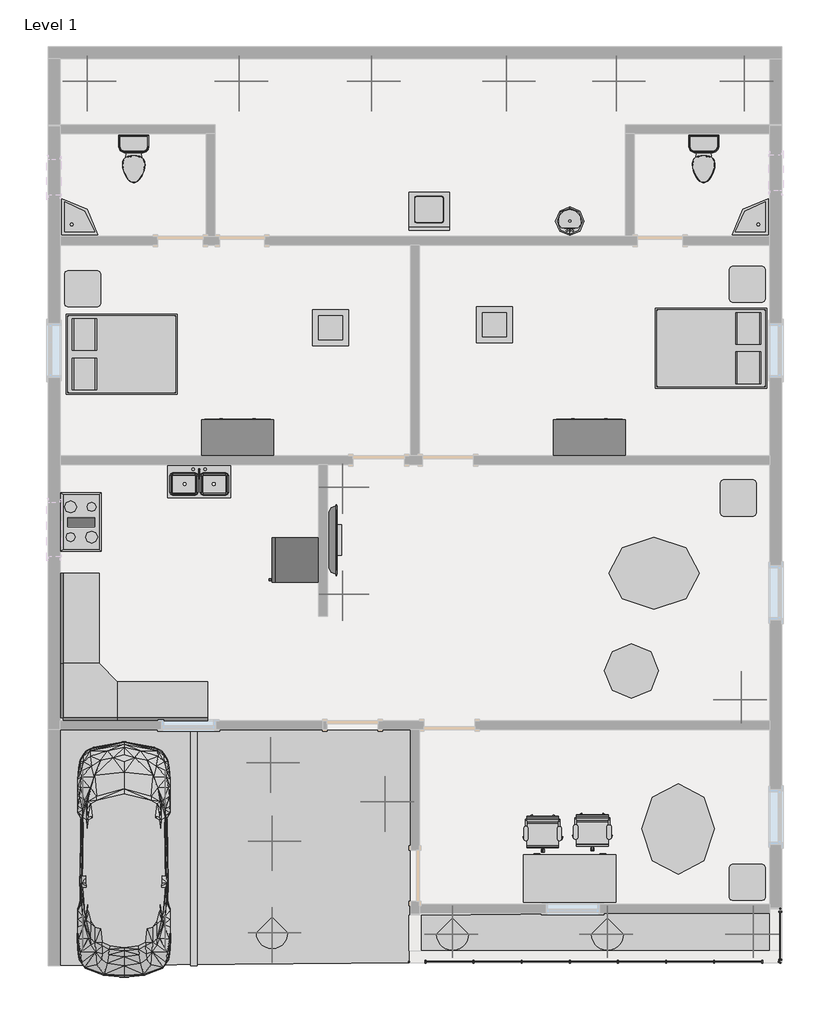
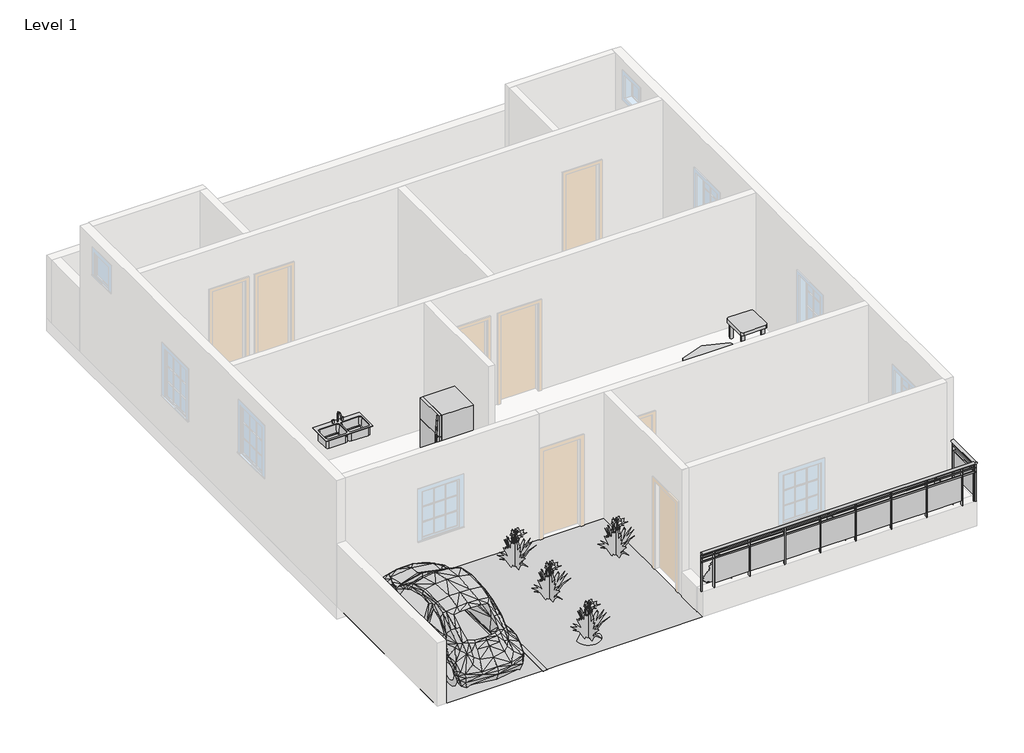
# One storey, part 2 of 2: 18 furniture elements, 16 geographic elements, 9 flow terminals, 7 proxies, 2 railings.
"""IFC4 building model written with IfcOpenShell, lengths in millimetres."""

from ifc_helpers import new_model, si_unit, point, frame, origin, place, context, project, spatial, polyline, ellipse_curve, trimmed, outline, extrude, triangles, transform, mapped, element, save
from ifc_brep_helpers import plane_surface, extruded_surface, advanced_brep
from components import proxy_bb1e6e30, m_rpc_beetle_m_rpc_beetle_b6d71803, parking_space_9_x_18_90_deg_c935943f, proxy_a13a33b2, proxy_718fa39f, flow_terminal_2b63360b, flow_terminal_accce45a, flow_terminal_bd5cdcf8, flow_terminal_a53be723, flow_terminal_d49f872f, toilet_domestic_3d_toilet_domestic_3d_f7549cf7, toilet_domestic_3d_toilet_domestic_3d_183bbd19, furniture_c8abb964, chair_task_arms_chair_task_arms_fa5a08ef, furniture_072f6425, furniture_9fa109b2, furniture_d9bcc661, furniture_b5c51a22, furniture_905aceb5, furniture_743965d2, furniture_5d68651d, furniture_45e3acac, rpc_plant_tropical_55f6ff97, rpc_plant_tropical_dagger_2_80c14bd7, rpc_plant_tropical_jungle_flame_3_9c4808c2

model = new_model("IFC4")

# Units and contexts
model_context = context("Model", 3, world=origin())
ifc_project = project(units=[si_unit("LENGTHUNIT", "METRE", prefix="MILLI")], contexts=[model_context])

# Site, building, storey
site = spatial("IfcSite", under=ifc_project)
building = spatial("IfcBuilding", under=site)
storey = spatial("IfcBuildingStorey", under=building, Name="Level 1", Elevation=0.0)

# Proxies
placement = place(None, origin())
element("IfcBuildingElementProxy", 1, Name="Building Element Proxy", at=placement, inside=storey, context=model_context, shape_type="Tessellation", body=[
    triangles([(-12787.9240906, 4557.2232857, 0.0), (-6666.5238968, 4557.2232857, 0.0), (-6679.223703, 620.2234068, 0.0), (-12787.9961792, 723.5583784, 0.0), (-7358.6740906, 4658.8234795, 0.0), (-6926.873703, 4658.8234795, 0.0), (-12584.723703, 569.4234189, 0.0)], [[4, 7, 1], [1, 7, 5], [3, 2, 5], [6, 5, 2], [3, 5, 7]], closed=False),
])
element("IfcBuildingElementProxy", 2, Name="Building Element Proxy", at=placement, inside=storey, context=model_context, shape_type="Tessellation", body=[
    triangles([(-6488.723703, 1420.3234795, 0.0), (-6488.723703, 823.423431, 0.0), (-595.9238726, 1458.4234795, 0.0), (-595.9238726, 823.423431, 0.0), (-3122.7224739, 1458.4234795, 0.0)], [[1, 2, 5], [5, 4, 3], [4, 5, 2]], closed=False),
])
proxy_shape = proxy_bb1e6e30(model_context)
element("IfcBuildingElementProxy", 3, Name="Cook Top-4 Unit : 36\" x 20\"", ObjectType="Cook Top-4 Unit : 36\" x 20\"", at=placement, inside=storey, context=model_context, shape_type="MappedRepresentation", body=[
    mapped(proxy_shape, transform((-12229.1238552, 8062.4234128, 0.0), x_axis=(0.0, 1.0000000000000002, 0.0), y_axis=(-1.0000000000000002, 0.0, 0.0), z_axis=(0.0, 0.0, 1.0))),
])
m_rpc_beetle_m_rpc_beetle_shape = m_rpc_beetle_m_rpc_beetle_b6d71803(model_context)
element("IfcBuildingElementProxy", 4, Name="M_RPC Beetle : M_RPC Beetle", ObjectType="M_RPC Beetle : M_RPC Beetle", at=placement, inside=storey, context=model_context, shape_type="MappedRepresentation", body=[
    mapped(m_rpc_beetle_m_rpc_beetle_shape, transform((-11505.2238552, 1128.2234128, 0.0), x_axis=(1.0, 0.0, 0.0), y_axis=(0.0, 1.0, 0.0), z_axis=(0.0, 0.0, 1.0))),
])
parking_space_9_x_18_90_deg_shape = parking_space_9_x_18_90_deg_c935943f(model_context)
element("IfcBuildingElementProxy", 5, Name="Parking Space : 9' x 18' - 90 deg", ObjectType="Parking Space : 9' x 18' - 90 deg", at=placement, inside=storey, context=model_context, shape_type="MappedRepresentation", body=[
    mapped(parking_space_9_x_18_90_deg_shape, transform((-10324.1238552, 569.4234128, 0.0), x_axis=(-1.0000000000000004, 0.0, 0.0), y_axis=(0.0, -1.0000000000000004, 0.0), z_axis=(0.0, 0.0, 1.0))),
])
proxy_2_shape = proxy_a13a33b2(model_context)
element("IfcBuildingElementProxy", 6, Name="Refrigerator : 30\" x 32\" RH", ObjectType="Refrigerator : 30\" x 32\" RH", at=placement, inside=storey, context=model_context, shape_type="MappedRepresentation", body=[
    mapped(proxy_2_shape, transform((-8588.9863552, 7419.8744413, 0.0), x_axis=(0.0, -1.0000000000000007, 0.0), y_axis=(1.0000000000000007, 0.0, 0.0), z_axis=(0.0, 0.0, 1.0))),
])
proxy_3_shape = proxy_718fa39f(model_context)
element("IfcBuildingElementProxy", 7, Name="Washer : 27\" x 25\" x 35\"", ObjectType="Washer : 27\" x 25\" x 35\"", at=placement, inside=storey, context=model_context, shape_type="MappedRepresentation", body=[
    mapped(proxy_3_shape, transform((-5931.2413237, 13587.173848, 0.0), x_axis=(-1.0000000000000004, 0.0, 0.0), y_axis=(0.0, -1.0000000000000004, 0.0), z_axis=(0.0, 0.0, 1.0))),
])

# Flow terminals
flow_terminal_shape = flow_terminal_2b63360b(model_context)
element("IfcFlowTerminal", 8, ObjectType="Floor Drain - Rectangular : 5\"x5\" Strainer - 2\" Drain", at=placement, inside=storey, context=model_context, shape_type="MappedRepresentation", body=[
    mapped(flow_terminal_shape, transform((-4710.7238552, 13066.2234128, 0.0), x_axis=(1.0, 0.0, 0.0), y_axis=(0.0, 1.0, 0.0), z_axis=(0.0, 0.0, 1.0))),
])
flow_terminal_2_shape = flow_terminal_accce45a(model_context)
element("IfcFlowTerminal", 9, ObjectType="Floor Drain - Round : 5\" Strainer - 2\" Drain", at=placement, inside=storey, context=model_context, shape_type="MappedRepresentation", body=[
    mapped(flow_terminal_2_shape, transform((-10425.7238552, 14361.6234128, 0.0), x_axis=(1.0, 0.0, 0.0), y_axis=(0.0, 1.0, 0.0), z_axis=(0.0, 0.0, 1.0))),
])
element("IfcFlowTerminal", 10, ObjectType="Floor Drain - Round : 5\" Strainer - 2\" Drain", at=placement, inside=storey, context=model_context, shape_type="MappedRepresentation", body=[
    mapped(flow_terminal_2_shape, transform((-2627.9238552, 14412.4234128, 0.0), x_axis=(1.0, 0.0, 0.0), y_axis=(0.0, 1.0, 0.0), z_axis=(0.0, 0.0, 1.0))),
])
flow_terminal_3_shape = flow_terminal_bd5cdcf8(model_context)
element("IfcFlowTerminal", 11, ObjectType="Sink - Corner Floor : 24\"", at=placement, inside=storey, context=model_context, shape_type="MappedRepresentation", body=[
    mapped(flow_terminal_3_shape, transform((-12559.3238552, 12913.8234128, 609.6), x_axis=(1.0, 0.0, 0.0), y_axis=(0.0, 1.0, 0.0), z_axis=(0.0, 0.0, 1.0))),
])
element("IfcFlowTerminal", 12, ObjectType="Sink - Corner Floor : 24\"", at=placement, inside=storey, context=model_context, shape_type="MappedRepresentation", body=[
    mapped(flow_terminal_3_shape, transform((-621.3238552, 12913.8234128, 609.6), x_axis=(0.0, 1.0, 0.0), y_axis=(-1.0, 0.0, 0.0), z_axis=(0.0, 0.0, 1.0))),
])
flow_terminal_4_shape = flow_terminal_a53be723(model_context)
element("IfcFlowTerminal", 13, ObjectType="Sink Kitchen-Double : 42\" x 21\"", at=placement, inside=storey, context=model_context, shape_type="MappedRepresentation", body=[
    mapped(flow_terminal_4_shape, transform((-10250.9130958, 8739.5280117, 0.0), x_axis=(1.0, 0.0, 0.0), y_axis=(0.0, 1.0, 0.0), z_axis=(0.0, 0.0, 1.0))),
])
flow_terminal_5_shape = flow_terminal_d49f872f(model_context)
element("IfcFlowTerminal", 14, ObjectType="Sink Vanity-Round : 19\" x 19\"", at=placement, inside=storey, context=model_context, shape_type="MappedRepresentation", body=[
    mapped(flow_terminal_5_shape, transform((-3877.4721147, 13227.1912438, 304.8), x_axis=(-1.0000000000000004, 0.0, 0.0), y_axis=(0.0, -1.0000000000000004, 0.0), z_axis=(0.0, 0.0, 1.0))),
])
toilet_domestic_3d_toilet_domestic_3d_shape = toilet_domestic_3d_toilet_domestic_3d_f7549cf7(model_context)
toilet_domestic_3d_toilet_domestic_3d_2_shape = toilet_domestic_3d_toilet_domestic_3d_183bbd19(model_context)
element("IfcFlowTerminal", 15, ObjectType="Toilet-Domestic-3D : Toilet-Domestic-3D", at=placement, inside=storey, context=model_context, shape_type="MappedRepresentation", body=[
    mapped(toilet_domestic_3d_toilet_domestic_3d_shape, transform((-11340.1238552, 14095.5273855, 0.0), x_axis=(1.0, 0.0, 0.0), y_axis=(0.0, 1.0, 0.0), z_axis=(0.0, 0.0, 1.0))),
    mapped(toilet_domestic_3d_toilet_domestic_3d_2_shape, transform((-11340.1238552, 14095.5273855, 0.0), x_axis=(1.0, 0.0, 0.0), y_axis=(0.0, 1.0, 0.0), z_axis=(0.0, 0.0, 1.0))),
])
element("IfcFlowTerminal", 16, ObjectType="Toilet-Domestic-3D : Toilet-Domestic-3D", at=placement, inside=storey, context=model_context, shape_type="MappedRepresentation", body=[
    mapped(toilet_domestic_3d_toilet_domestic_3d_shape, transform((-1713.5238552, 14095.5273855, 0.0), x_axis=(1.0, 0.0, 0.0), y_axis=(0.0, 1.0, 0.0), z_axis=(0.0, 0.0, 1.0))),
    mapped(toilet_domestic_3d_toilet_domestic_3d_2_shape, transform((-1713.5238552, 14095.5273855, 0.0), x_axis=(1.0, 0.0, 0.0), y_axis=(0.0, 1.0, 0.0), z_axis=(0.0, 0.0, 1.0))),
])

# Furniture
furniture_shape = furniture_c8abb964(model_context)
element("IfcFurniture", 17, ObjectType="Bed-Box : Double 53\" x 74\"", at=placement, inside=storey, context=model_context, shape_type="MappedRepresentation", body=[
    mapped(furniture_shape, transform((-11777.7533634, 10555.3709538, 0.0), x_axis=(0.0, 1.0, 0.0), y_axis=(-1.0, 0.0, 0.0), z_axis=(0.0, 0.0, 1.0))),
])
element("IfcFurniture", 18, ObjectType="Bed-Box : Double 53\" x 74\"", at=placement, inside=storey, context=model_context, shape_type="MappedRepresentation", body=[
    mapped(furniture_shape, transform((-1352.094347, 11335.2758718, 0.0), x_axis=(0.0, -1.0, 0.0), y_axis=(1.0, 0.0, 0.0), z_axis=(0.0, 0.0, 1.0))),
])
chair_task_arms_chair_task_arms_shape = chair_task_arms_chair_task_arms_fa5a08ef(model_context)
element("IfcFurniture", 19, ObjectType="Chair-Task Arms : Chair-Task Arms", at=placement, inside=storey, context=model_context, shape_type="MappedRepresentation", body=[
    mapped(chair_task_arms_chair_task_arms_shape, transform((-4290.3330355, 2848.9693144, 0.0), x_axis=(-1.000000000000001, 0.0, 0.0), y_axis=(0.0, -1.000000000000001, 0.0), z_axis=(0.0, 0.0, 1.0))),
])
element("IfcFurniture", 20, ObjectType="Chair-Task Arms : Chair-Task Arms", at=placement, inside=storey, context=model_context, shape_type="MappedRepresentation", body=[
    mapped(chair_task_arms_chair_task_arms_shape, transform((-3452.1330355, 2874.3693144, 0.0), x_axis=(-1.0000000000000007, 0.0, 0.0), y_axis=(0.0, -1.0000000000000007, 0.0), z_axis=(0.0, 0.0, 1.0))),
])
furniture_2_shape = furniture_072f6425(model_context)
element("IfcFurniture", 21, ObjectType="Desk : 60\" x 30\" Student", at=placement, inside=storey, context=model_context, shape_type="MappedRepresentation", body=[
    mapped(furniture_2_shape, transform((-4736.1238552, 1661.6234128, 0.0), x_axis=(1.0000000000000009, 0.0, 0.0), y_axis=(0.0, 1.0000000000000009, 0.0), z_axis=(0.0, 0.0, 1.0))),
])
furniture_3_shape = furniture_9fa109b2(model_context)
element("IfcFurniture", 22, ObjectType="Dresser : 48\" x 72\" x 24\"", at=placement, inside=storey, context=model_context, shape_type="MappedRepresentation", body=[
    mapped(furniture_3_shape, transform((-9856.7171151, 9121.6604587, 0.0), x_axis=(-1.0000000000000004, 0.0, 0.0), y_axis=(0.0, -1.0000000000000004, 0.0), z_axis=(0.0, 0.0, 1.0))),
])
element("IfcFurniture", 23, ObjectType="Dresser : 48\" x 72\" x 24\"", at=placement, inside=storey, context=model_context, shape_type="MappedRepresentation", body=[
    mapped(furniture_3_shape, transform((-3913.1171151, 9121.6604587, 0.0), x_axis=(-1.0000000000000004, 0.0, 0.0), y_axis=(0.0, -1.0000000000000004, 0.0), z_axis=(0.0, 0.0, 1.0))),
])
furniture_4_shape = furniture_d9bcc661(model_context)
element("IfcFurniture", 24, ObjectType="TV - Flat Screen : 46\"", at=placement, inside=storey, context=model_context, shape_type="MappedRepresentation", body=[
    mapped(furniture_4_shape, transform((-7978.3782681, 7761.567927, 914.4), x_axis=(0.0, 1.0000000000000002, 0.0), y_axis=(-1.0000000000000002, 0.0, 0.0), z_axis=(0.0, 0.0, 1.0))),
])
furniture_5_shape = furniture_b5c51a22(model_context)
element("IfcFurniture", 25, ObjectType="Table-Coffee : 24\" x 24\" x 24\"", at=placement, inside=storey, context=model_context, shape_type="MappedRepresentation", body=[
    mapped(furniture_5_shape, transform((-8030.9896219, 11243.812335, 0.0), x_axis=(1.0, 0.0, 0.0), y_axis=(0.0, 1.0, 0.0), z_axis=(0.0, 0.0, 1.0))),
])
element("IfcFurniture", 26, ObjectType="Table-Coffee : 24\" x 24\" x 24\"", at=placement, inside=storey, context=model_context, shape_type="MappedRepresentation", body=[
    mapped(furniture_5_shape, transform((-5262.3896219, 11294.612335, 0.0), x_axis=(1.0, 0.0, 0.0), y_axis=(0.0, 1.0, 0.0), z_axis=(0.0, 0.0, 1.0))),
])
furniture_6_shape = furniture_905aceb5(model_context)
element("IfcFurniture", 27, ObjectType="Table-Dining Round w Chairs : 36\" Diameter", at=placement, inside=storey, context=model_context, shape_type="MappedRepresentation", body=[
    mapped(furniture_6_shape, transform((-3036.4058224, 5732.7021013, 0.0), x_axis=(1.0, 0.0, 0.0), y_axis=(0.0, 1.0, 0.0), z_axis=(0.0, 0.0, 1.0))),
])
furniture_7_shape = furniture_743965d2(model_context)
element("IfcFurniture", 28, ObjectType="Table-Ellipse : 60\" x 48\"", at=placement, inside=storey, context=model_context, shape_type="MappedRepresentation", body=[
    mapped(furniture_7_shape, transform((-2145.3238552, 2880.8234128, 0.0), x_axis=(0.0, -1.0000000000000004, 0.0), y_axis=(1.0000000000000004, 0.0, 0.0), z_axis=(0.0, 0.0, 1.0))),
])
element("IfcFurniture", 29, ObjectType="Table-Ellipse : 60\" x 48\"", at=placement, inside=storey, context=model_context, shape_type="MappedRepresentation", body=[
    mapped(furniture_7_shape, transform((-2551.7238552, 7198.8234128, 0.0), x_axis=(1.0, 0.0, 0.0), y_axis=(0.0, 1.0, 0.0), z_axis=(0.0, 0.0, 1.0))),
])
furniture_8_shape = furniture_5d68651d(model_context)
element("IfcFurniture", 30, ObjectType="Table-End : 24\" x 24\"", at=placement, inside=storey, context=model_context, shape_type="MappedRepresentation", body=[
    mapped(furniture_8_shape, transform((-12512.2574855, 11847.0234128, 0.0), x_axis=(1.0, 0.0, 0.0), y_axis=(0.0, 1.0, 0.0), z_axis=(0.0, 0.0, 1.0))),
])
element("IfcFurniture", 31, ObjectType="Table-End : 24\" x 24\"", at=placement, inside=storey, context=model_context, shape_type="MappedRepresentation", body=[
    mapped(furniture_8_shape, transform((-1285.4574855, 11923.2234128, 0.0), x_axis=(1.0, 0.0, 0.0), y_axis=(0.0, 1.0, 0.0), z_axis=(0.0, 0.0, 1.0))),
])
element("IfcFurniture", 32, ObjectType="Table-End : 24\" x 24\"", at=placement, inside=storey, context=model_context, shape_type="MappedRepresentation", body=[
    mapped(furniture_8_shape, transform((-1437.8574855, 8316.4234128, 0.0), x_axis=(1.0, 0.0, 0.0), y_axis=(0.0, 1.0, 0.0), z_axis=(0.0, 0.0, 1.0))),
])
element("IfcFurniture", 33, ObjectType="Table-End : 24\" x 24\"", at=placement, inside=storey, context=model_context, shape_type="MappedRepresentation", body=[
    mapped(furniture_8_shape, transform((-1285.4574855, 1826.7234128, 0.0), x_axis=(1.0, 0.0, 0.0), y_axis=(0.0, 1.0, 0.0), z_axis=(0.0, 0.0, 1.0))),
])
furniture_9_shape = furniture_45e3acac(model_context)
element("IfcFurniture", 34, ObjectType="Work Station Cubicle : 96\" x 96\"", at=placement, inside=storey, context=model_context, shape_type="MappedRepresentation", body=[
    mapped(furniture_9_shape, transform((-13079.7468628, 4841.355165, 0.0), x_axis=(0.0, 1.0000000000000002, 0.0), y_axis=(-1.0000000000000002, 0.0, 0.0), z_axis=(0.0, 0.0, 1.0))),
])

# Geographic elements
rpc_plant_tropical_shape = rpc_plant_tropical_55f6ff97(model_context)
element("IfcGeographicElement", 35, ObjectType="RPC Plant - Tropical", at=placement, inside=storey, context=model_context, shape_type="MappedRepresentation", body=[
    mapped(rpc_plant_tropical_shape, transform((-12127.5238552, 15504.6234128, 0.0), x_axis=(1.0, 0.0, 0.0), y_axis=(0.0, 1.0, 0.0), z_axis=(0.0, 0.0, 1.0))),
])
element("IfcGeographicElement", 36, ObjectType="RPC Plant - Tropical", at=placement, inside=storey, context=model_context, shape_type="MappedRepresentation", body=[
    mapped(rpc_plant_tropical_shape, transform((-9562.1238552, 15504.6234128, 0.0), x_axis=(1.0, 0.0, 0.0), y_axis=(0.0, 1.0, 0.0), z_axis=(0.0, 0.0, 1.0))),
])
element("IfcGeographicElement", 37, ObjectType="RPC Plant - Tropical", at=placement, inside=storey, context=model_context, shape_type="MappedRepresentation", body=[
    mapped(rpc_plant_tropical_shape, transform((-7326.9238552, 15504.6234128, 0.0), x_axis=(1.0, 0.0, 0.0), y_axis=(0.0, 1.0, 0.0), z_axis=(0.0, 0.0, 1.0))),
])
element("IfcGeographicElement", 38, ObjectType="RPC Plant - Tropical", at=placement, inside=storey, context=model_context, shape_type="MappedRepresentation", body=[
    mapped(rpc_plant_tropical_shape, transform((-5040.9238552, 15504.6234128, 0.0), x_axis=(1.0, 0.0, 0.0), y_axis=(0.0, 1.0, 0.0), z_axis=(0.0, 0.0, 1.0))),
])
element("IfcGeographicElement", 39, ObjectType="RPC Plant - Tropical", at=placement, inside=storey, context=model_context, shape_type="MappedRepresentation", body=[
    mapped(rpc_plant_tropical_shape, transform((-3186.7238552, 15504.6234128, 0.0), x_axis=(1.0, 0.0, 0.0), y_axis=(0.0, 1.0, 0.0), z_axis=(0.0, 0.0, 1.0))),
])
element("IfcGeographicElement", 40, ObjectType="RPC Plant - Tropical", at=placement, inside=storey, context=model_context, shape_type="MappedRepresentation", body=[
    mapped(rpc_plant_tropical_shape, transform((-1027.7238552, 15504.6234128, 0.0), x_axis=(1.0, 0.0, 0.0), y_axis=(0.0, 1.0, 0.0), z_axis=(0.0, 0.0, 1.0))),
])
element("IfcGeographicElement", 41, ObjectType="RPC Plant - Tropical", at=placement, inside=storey, context=model_context, shape_type="MappedRepresentation", body=[
    mapped(rpc_plant_tropical_shape, transform((-7098.3238552, 3338.0234128, 0.0), x_axis=(1.0, 0.0, 0.0), y_axis=(0.0, 1.0, 0.0), z_axis=(0.0, 0.0, 1.0))),
])
element("IfcGeographicElement", 42, ObjectType="RPC Plant - Tropical", at=placement, inside=storey, context=model_context, shape_type="MappedRepresentation", body=[
    mapped(rpc_plant_tropical_shape, transform((-9028.7238552, 3998.4234128, 0.0), x_axis=(1.0, 0.0, 0.0), y_axis=(0.0, 1.0, 0.0), z_axis=(0.0, 0.0, 1.0))),
])
element("IfcGeographicElement", 43, ObjectType="RPC Plant - Tropical", at=placement, inside=storey, context=model_context, shape_type="MappedRepresentation", body=[
    mapped(rpc_plant_tropical_shape, transform((-9003.3238552, 1128.2234128, 0.0), x_axis=(1.0, 0.0, 0.0), y_axis=(0.0, 1.0, 0.0), z_axis=(0.0, 0.0, 1.0))),
])
element("IfcGeographicElement", 44, ObjectType="RPC Plant - Tropical", at=placement, inside=storey, context=model_context, shape_type="MappedRepresentation", body=[
    mapped(rpc_plant_tropical_shape, transform((-9003.3238552, 2677.6234128, 0.0), x_axis=(1.0, 0.0, 0.0), y_axis=(0.0, 1.0, 0.0), z_axis=(0.0, 0.0, 1.0))),
])
rpc_plant_tropical_dagger_2_shape = rpc_plant_tropical_dagger_2_80c14bd7(model_context)
element("IfcGeographicElement", 45, ObjectType="RPC Plant - Tropical : Dagger - 2'", at=placement, inside=storey, context=model_context, shape_type="MappedRepresentation", body=[
    mapped(rpc_plant_tropical_dagger_2_shape, transform((-7809.5238552, 6843.2234128, 0.0), x_axis=(1.0, 0.0, 0.0), y_axis=(0.0, 1.0, 0.0), z_axis=(0.0, 0.0, 1.0))),
])
element("IfcGeographicElement", 46, ObjectType="RPC Plant - Tropical : Dagger - 2'", at=placement, inside=storey, context=model_context, shape_type="MappedRepresentation", body=[
    mapped(rpc_plant_tropical_dagger_2_shape, transform((-7809.5238552, 8646.6234128, 0.0), x_axis=(1.0, 0.0, 0.0), y_axis=(0.0, 1.0, 0.0), z_axis=(0.0, 0.0, 1.0))),
])
rpc_plant_tropical_jungle_flame_3_shape = rpc_plant_tropical_jungle_flame_3_9c4808c2(model_context)
element("IfcGeographicElement", 47, ObjectType="RPC Plant - Tropical : Jungle Flame - 3'", at=placement, inside=storey, context=model_context, shape_type="MappedRepresentation", body=[
    mapped(rpc_plant_tropical_jungle_flame_3_shape, transform((-1078.5238552, 5065.2234128, 0.0), x_axis=(1.0, 0.0, 0.0), y_axis=(0.0, 1.0, 0.0), z_axis=(0.0, 0.0, 1.0))),
])
element("IfcGeographicElement", 48, ObjectType="RPC Plant - Tropical : Jungle Flame - 3'", at=placement, inside=storey, context=model_context, shape_type="MappedRepresentation", body=[
    mapped(rpc_plant_tropical_jungle_flame_3_shape, transform((-5955.3238552, 1102.8234128, 0.0), x_axis=(1.0, 0.0, 0.0), y_axis=(0.0, 1.0, 0.0), z_axis=(0.0, 0.0, 1.0))),
])
element("IfcGeographicElement", 49, ObjectType="RPC Plant - Tropical : Jungle Flame - 3'", at=placement, inside=storey, context=model_context, shape_type="MappedRepresentation", body=[
    mapped(rpc_plant_tropical_jungle_flame_3_shape, transform((-875.3238552, 1102.8234128, 0.0), x_axis=(1.0, 0.0, 0.0), y_axis=(0.0, 1.0, 0.0), z_axis=(0.0, 0.0, 1.0))),
])
element("IfcGeographicElement", 50, ObjectType="RPC Plant - Tropical : Jungle Flame - 3'", at=placement, inside=storey, context=model_context, shape_type="MappedRepresentation", body=[
    mapped(rpc_plant_tropical_jungle_flame_3_shape, transform((-3339.1238552, 1102.8234128, 0.0), x_axis=(1.0, 0.0, 0.0), y_axis=(0.0, 1.0, 0.0), z_axis=(0.0, 0.0, 1.0))),
])

# Railings
element("IfcRailing", 51, ObjectType="Glass Panel - Bottom Fill", at=placement, inside=storey, context=model_context, shape_type="SolidModel", body=[
    advanced_brep(
    [(-6691.9238552, 677.3734128, 1524.0), (-6691.9238552, 601.1734128, 1524.0), (-443.5238552, 677.3734128, 1524.0), (-443.5238552, 601.1734128, 1524.0)],
    [
        (0, 1, ellipse_curve(frame((-6691.9238552, 639.2734128, 1524.0), z_axis=(-1.0, 0.0, 0.0), x_axis=(0.0, -1.0, 0.0)), 38.1, 28.575)),
        (1, 0, ellipse_curve(frame((-6691.9238552, 639.2734128, 1524.0), z_axis=(-1.0, 0.0, 0.0), x_axis=(0.0, -1.0, 0.0)), 38.1, 28.575)),
        (2, 3, ellipse_curve(frame((-443.5238552, 639.2734128, 1524.0), z_axis=(1.0, 0.0, 0.0), x_axis=(0.0, -1.0, 0.0)), 38.1, 28.575)),
        (3, 2, ellipse_curve(frame((-443.5238552, 639.2734128, 1524.0), z_axis=(1.0, 0.0, 0.0), x_axis=(0.0, -1.0, 0.0)), 38.1, 28.575)),
        (0, 2),
        (3, 1),
    ],
    [
        plane_surface(frame((-6691.9238552, 639.2734128, 1524.0), z_axis=(-1.0, 0.0, 0.0), x_axis=(0.0, 1.0, 0.0))),
        plane_surface(frame((-443.5238552, 639.2734128, 1524.0), z_axis=(1.0, 0.0, 0.0), x_axis=(0.0, 1.0, 0.0))),
        extruded_surface(trimmed(ellipse_curve(frame((-443.5238552, 639.2734128, 1524.0), z_axis=(-1.0, 0.0, 0.0), x_axis=(0.0, -1.0, 0.0)), 38.1, 28.575), [point((-443.5238552, 677.3734128, 1524.0))], [point((-443.5238552, 601.1734128, 1524.0))], True, "CARTESIAN"), (-6248.4, 0.0, 0.0), 6248.4),
        extruded_surface(trimmed(ellipse_curve(frame((-443.5238552, 639.2734128, 1524.0), z_axis=(-1.0, 0.0, 0.0), x_axis=(0.0, -1.0, 0.0)), 38.1, 28.575), [point((-443.5238552, 601.1734128, 1524.0))], [point((-443.5238552, 677.3734128, 1524.0))], True, "CARTESIAN"), (-6248.4, 0.0, 0.0), 6248.4),
    ],
    [
        (0, [[1, 2]]),
        (1, [[3, 4]]),
        (2, [[-1, 5, -4, 6]]),
        (3, [[-2, -6, -3, -5]]),
    ],
),
    extrude(outline(polyline([(-6691.9238552, 626.5734128), (-6691.9238552, 651.9734128), (-443.5238552, 651.9734128), (-443.5238552, 626.5734128), (-6691.9238552, 626.5734128)])), frame((0.0, 0.0, 1409.7), z_axis=(0.0, 0.0, 1.0), x_axis=(1.0, 0.0, 0.0)), (0.0, 0.0, 1.0), 25.4),
    extrude(outline(polyline([(-6691.9238552, 626.5734128), (-6691.9238552, 651.9734128), (-443.5238552, 651.9734128), (-443.5238552, 626.5734128), (-6691.9238552, 626.5734128)])), frame((0.0, 0.0, 1308.1), z_axis=(0.0, 0.0, 1.0), x_axis=(1.0, 0.0, 0.0)), (0.0, 0.0, 1.0), 25.4),
    extrude(outline(polyline([(-729.2738552, 613.8734128), (-729.2738552, 664.6734128), (-716.5738552, 664.6734128), (-716.5738552, 613.8734128), (-729.2738552, 613.8734128)])), frame((0.0, 0.0, 609.6), z_axis=(0.0, 0.0, 1.0), x_axis=(1.0, 0.0, 0.0)), (0.0, 0.0, 1.0), 885.6788223),
    extrude(outline(polyline([(-1535.7238552, 645.8085698), (-722.9238552, 645.8085698), (-722.9238552, 639.4585698), (-1535.7238552, 639.4585698), (-1535.7238552, 645.8085698)])), frame((0.0, 0.0, 711.2), z_axis=(0.0, 0.0, 1.0), x_axis=(1.0, 0.0, 0.0)), (0.0, 0.0, 1.0), 596.9),
    extrude(outline(polyline([(-1542.0738552, 613.8734128), (-1542.0738552, 664.6734128), (-1529.3738552, 664.6734128), (-1529.3738552, 613.8734128), (-1542.0738552, 613.8734128)])), frame((0.0, 0.0, 609.6), z_axis=(0.0, 0.0, 1.0), x_axis=(1.0, 0.0, 0.0)), (0.0, 0.0, 1.0), 885.6788223),
    extrude(outline(polyline([(-2348.5238552, 645.8085698), (-1535.7238552, 645.8085698), (-1535.7238552, 639.4585698), (-2348.5238552, 639.4585698), (-2348.5238552, 645.8085698)])), frame((0.0, 0.0, 711.2), z_axis=(0.0, 0.0, 1.0), x_axis=(1.0, 0.0, 0.0)), (0.0, 0.0, 1.0), 596.9),
    extrude(outline(polyline([(-2354.8738552, 613.8734128), (-2354.8738552, 664.6734128), (-2342.1738552, 664.6734128), (-2342.1738552, 613.8734128), (-2354.8738552, 613.8734128)])), frame((0.0, 0.0, 609.6), z_axis=(0.0, 0.0, 1.0), x_axis=(1.0, 0.0, 0.0)), (0.0, 0.0, 1.0), 885.6788223),
    extrude(outline(polyline([(-3161.3238552, 645.8085698), (-2348.5238552, 645.8085698), (-2348.5238552, 639.4585698), (-3161.3238552, 639.4585698), (-3161.3238552, 645.8085698)])), frame((0.0, 0.0, 711.2), z_axis=(0.0, 0.0, 1.0), x_axis=(1.0, 0.0, 0.0)), (0.0, 0.0, 1.0), 596.9),
    extrude(outline(polyline([(-3167.6738552, 613.8734128), (-3167.6738552, 664.6734128), (-3154.9738552, 664.6734128), (-3154.9738552, 613.8734128), (-3167.6738552, 613.8734128)])), frame((0.0, 0.0, 609.6), z_axis=(0.0, 0.0, 1.0), x_axis=(1.0, 0.0, 0.0)), (0.0, 0.0, 1.0), 885.6788223),
    extrude(outline(polyline([(-3974.1238552, 645.8085698), (-3161.3238552, 645.8085698), (-3161.3238552, 639.4585698), (-3974.1238552, 639.4585698), (-3974.1238552, 645.8085698)])), frame((0.0, 0.0, 711.2), z_axis=(0.0, 0.0, 1.0), x_axis=(1.0, 0.0, 0.0)), (0.0, 0.0, 1.0), 596.9),
    extrude(outline(polyline([(-3980.4738552, 613.8734128), (-3980.4738552, 664.6734128), (-3967.7738552, 664.6734128), (-3967.7738552, 613.8734128), (-3980.4738552, 613.8734128)])), frame((0.0, 0.0, 609.6), z_axis=(0.0, 0.0, 1.0), x_axis=(1.0, 0.0, 0.0)), (0.0, 0.0, 1.0), 885.6788223),
    extrude(outline(polyline([(-4786.9238552, 645.8085698), (-3974.1238552, 645.8085698), (-3974.1238552, 639.4585698), (-4786.9238552, 639.4585698), (-4786.9238552, 645.8085698)])), frame((0.0, 0.0, 711.2), z_axis=(0.0, 0.0, 1.0), x_axis=(1.0, 0.0, 0.0)), (0.0, 0.0, 1.0), 596.9),
    extrude(outline(polyline([(-4793.2738552, 613.8734128), (-4793.2738552, 664.6734128), (-4780.5738552, 664.6734128), (-4780.5738552, 613.8734128), (-4793.2738552, 613.8734128)])), frame((0.0, 0.0, 609.6), z_axis=(0.0, 0.0, 1.0), x_axis=(1.0, 0.0, 0.0)), (0.0, 0.0, 1.0), 885.6788223),
    extrude(outline(polyline([(-5599.7238552, 645.8085698), (-4786.9238552, 645.8085698), (-4786.9238552, 639.4585698), (-5599.7238552, 639.4585698), (-5599.7238552, 645.8085698)])), frame((0.0, 0.0, 711.2), z_axis=(0.0, 0.0, 1.0), x_axis=(1.0, 0.0, 0.0)), (0.0, 0.0, 1.0), 596.9),
    extrude(outline(polyline([(-5606.0738552, 613.8734128), (-5606.0738552, 664.6734128), (-5593.3738552, 664.6734128), (-5593.3738552, 613.8734128), (-5606.0738552, 613.8734128)])), frame((0.0, 0.0, 609.6), z_axis=(0.0, 0.0, 1.0), x_axis=(1.0, 0.0, 0.0)), (0.0, 0.0, 1.0), 885.6788223),
    extrude(outline(polyline([(-6412.5238552, 645.8085698), (-5599.7238552, 645.8085698), (-5599.7238552, 639.4585698), (-6412.5238552, 639.4585698), (-6412.5238552, 645.8085698)])), frame((0.0, 0.0, 711.2), z_axis=(0.0, 0.0, 1.0), x_axis=(1.0, 0.0, 0.0)), (0.0, 0.0, 1.0), 596.9),
    extrude(outline(polyline([(-6418.8738552, 613.8734128), (-6418.8738552, 664.6734128), (-6406.1738552, 664.6734128), (-6406.1738552, 613.8734128), (-6418.8738552, 613.8734128)])), frame((0.0, 0.0, 609.6), z_axis=(0.0, 0.0, 1.0), x_axis=(1.0, 0.0, 0.0)), (0.0, 0.0, 1.0), 885.6788223),
    extrude(outline(polyline([(-456.2238552, 629.7484128), (-456.2238552, 648.7984128), (-437.1738552, 648.7984128), (-437.1738552, 629.7484128), (-456.2238552, 629.7484128)])), frame((0.0, 0.0, 609.6), z_axis=(0.0, 0.0, 1.0), x_axis=(1.0, 0.0, 0.0)), (0.0, 0.0, 1.0), 885.6788223),
    extrude(outline(polyline([(-6698.2738552, 629.7484128), (-6698.2738552, 648.7984128), (-6679.2238552, 648.7984128), (-6679.2238552, 629.7484128), (-6698.2738552, 629.7484128)])), frame((0.0, 0.0, 609.6), z_axis=(0.0, 0.0, 1.0), x_axis=(1.0, 0.0, 0.0)), (0.0, 0.0, 1.0), 885.6788223),
])
element("IfcRailing", 52, ObjectType="Glass Panel - Bottom Fill", at=placement, inside=storey, context=model_context, shape_type="SolidModel", body=[
    advanced_brep(
    [(-456.2238552, 620.2234128, 1524.0), (-380.0238552, 620.2234128, 1524.0), (-456.2238552, 1534.6234128, 1524.0), (-380.0238552, 1534.6234128, 1524.0)],
    [
        (0, 1, ellipse_curve(frame((-418.1238552, 620.2234128, 1524.0), z_axis=(0.0, -1.0, 0.0), x_axis=(1.0, 0.0, 0.0)), 38.1, 28.575)),
        (1, 0, ellipse_curve(frame((-418.1238552, 620.2234128, 1524.0), z_axis=(0.0, -1.0, 0.0), x_axis=(1.0, 0.0, 0.0)), 38.1, 28.575)),
        (2, 3, ellipse_curve(frame((-418.1238552, 1534.6234128, 1524.0), z_axis=(0.0, 1.0, 0.0), x_axis=(1.0, 0.0, 0.0)), 38.1, 28.575)),
        (3, 2, ellipse_curve(frame((-418.1238552, 1534.6234128, 1524.0), z_axis=(0.0, 1.0, 0.0), x_axis=(1.0, 0.0, 0.0)), 38.1, 28.575)),
        (0, 2),
        (3, 1),
    ],
    [
        plane_surface(frame((-418.1238552, 620.2234128, 1524.0), z_axis=(0.0, -1.0, 0.0), x_axis=(0.0, 0.0, 1.0))),
        plane_surface(frame((-418.1238552, 1534.6234128, 1524.0), z_axis=(0.0, 1.0, 0.0), x_axis=(0.0, 0.0, 1.0))),
        extruded_surface(trimmed(ellipse_curve(frame((-418.1238552, 1534.6234128, 1524.0), z_axis=(0.0, -1.0, 0.0), x_axis=(1.0, 0.0, 0.0)), 38.1, 28.575), [point((-456.2238552, 1534.6234128, 1524.0))], [point((-380.0238552, 1534.6234128, 1524.0))], True, "CARTESIAN"), (0.0, -914.4000000000001, 0.0), 914.4000000000001),
        extruded_surface(trimmed(ellipse_curve(frame((-418.1238552, 1534.6234128, 1524.0), z_axis=(0.0, -1.0, 0.0), x_axis=(1.0, 0.0, 0.0)), 38.1, 28.575), [point((-380.0238552, 1534.6234128, 1524.0))], [point((-456.2238552, 1534.6234128, 1524.0))], True, "CARTESIAN"), (0.0, -914.4000000000001, 0.0), 914.4000000000001),
    ],
    [
        (0, [[1, 2]]),
        (1, [[3, 4]]),
        (2, [[-1, 5, -4, 6]]),
        (3, [[-2, -6, -3, -5]]),
    ],
),
    extrude(outline(polyline([(-405.4238552, 620.2234128), (-430.8238552, 620.2234128), (-430.8238552, 1534.6234128), (-405.4238552, 1534.6234128), (-405.4238552, 620.2234128)])), frame((0.0, 0.0, 1409.7), z_axis=(0.0, 0.0, 1.0), x_axis=(1.0, 0.0, 0.0)), (0.0, 0.0, 1.0), 25.4),
    extrude(outline(polyline([(-405.4238552, 620.2234128), (-430.8238552, 620.2234128), (-430.8238552, 1534.6234128), (-405.4238552, 1534.6234128), (-405.4238552, 620.2234128)])), frame((0.0, 0.0, 1308.1), z_axis=(0.0, 0.0, 1.0), x_axis=(1.0, 0.0, 0.0)), (0.0, 0.0, 1.0), 25.4),
    extrude(outline(polyline([(-392.7238552, 1477.4734128), (-443.5238552, 1477.4734128), (-443.5238552, 1490.1734128), (-392.7238552, 1490.1734128), (-392.7238552, 1477.4734128)])), frame((0.0, 0.0, 609.6), z_axis=(0.0, 0.0, 1.0), x_axis=(1.0, 0.0, 0.0)), (0.0, 0.0, 1.0), 885.6788223),
    extrude(outline(polyline([(-424.6590122, 671.0234128), (-424.6590122, 1483.8234128), (-418.3090122, 1483.8234128), (-418.3090122, 671.0234128), (-424.6590122, 671.0234128)])), frame((0.0, 0.0, 711.2), z_axis=(0.0, 0.0, 1.0), x_axis=(1.0, 0.0, 0.0)), (0.0, 0.0, 1.0), 596.9),
    extrude(outline(polyline([(-392.7238552, 664.6734128), (-443.5238552, 664.6734128), (-443.5238552, 677.3734128), (-392.7238552, 677.3734128), (-392.7238552, 664.6734128)])), frame((0.0, 0.0, 609.6), z_axis=(0.0, 0.0, 1.0), x_axis=(1.0, 0.0, 0.0)), (0.0, 0.0, 1.0), 885.6788223),
    extrude(outline(polyline([(-408.5988552, 1521.9234128), (-427.6488552, 1521.9234128), (-427.6488552, 1540.9734128), (-408.5988552, 1540.9734128), (-408.5988552, 1521.9234128)])), frame((0.0, 0.0, 609.6), z_axis=(0.0, 0.0, 1.0), x_axis=(1.0, 0.0, 0.0)), (0.0, 0.0, 1.0), 885.6788223),
    extrude(outline(polyline([(-408.5988552, 613.8734128), (-427.6488552, 613.8734128), (-427.6488552, 632.9234128), (-408.5988552, 632.9234128), (-408.5988552, 613.8734128)])), frame((0.0, 0.0, 609.6), z_axis=(0.0, 0.0, 1.0), x_axis=(1.0, 0.0, 0.0)), (0.0, 0.0, 1.0), 885.6788223),
])

save(model, "model.ifc")

# Revit data of these elements
# Type "Cook Top-4 Unit : 36\" x 20\""
#   Assembly Code = "E1090400"
#   Depth = 2' - 0"
#   Width = 3' - 0"
#   Burner Material = Steel, Chrome Plated
#   Cooktop Material = Steel, Polished
#   Default Elevation = 0
# Type "M_RPC Beetle : M_RPC Beetle"
#   built-in parameter 1005198 = "{2, 15},{39, RPC-16-0U6E-L4EG-ENH1-J3KF-SVEL-0TX4-C0},{1, 0},{1, 0},{2, 18},{1, 8},{5, Color},{1, 0},{1, 0},{3, 0.8},{3, 0.8},{3, 0.8},{1, 8},{7, BBoxMin},{1, 0},{1, 0},{1, 0},{1, 0},{1, 0},{1, 8},{7, BBoxMax},{1, 0},{1, 0},{1, 0},{1, 0},{1, 0},{2, 11},{9, RPCTypeId},{1, 0},{1, 0},{39, RPC-16-0U6E-L4EG-ENH1-J3KF-SVEL-0TX4-C0},{1, 6},{14, RPCPlantHeight},{1, 0},{1, 0},{4, 4.92},{2, 11},{7, keyword},{1, 0},{1, 0},{39, :RPCs:Auto_Economy/Midsize:Geometry:RPC},{2, 11},{8, category},{1, 0},{1, 0},{20, Auto_Economy/Midsize},{2, 11},{12, LocalizedUID},{1, 0},{1, 0},{13, VW Beetle [4]},{2, 14},{6, Height},{1, 0},{1, 0},{4, 4.92},{1, 2},{16, Cast Reflections},{1, 0},{1, 0},{1, 0},{1, 4},{12, Transparency},{1, 0},{1, 0},{2, 18},{1, 4},{7, Tinting},{1, 0},{1, 0},{2, 50},{1, 2},{11, Use Tinting},{1, 0},{1, 0},{1, 0},{1, 2},{13, License Plate},{1, 0},{1, 0},{1, 0},{2, 11},{21, License Plate Texture},{1, 0},{1, 0},{64, __RPC:/object data/textures/car/plate/textures/default/rgb/0/0/0},{2, 11},{23, i_License Plate Texture},{1, 0},{1, 0},{0, },{1, 2},{12, Custom Plate},{1, 0},{1, 0},{1, 0},{2, 11},{23, License Plate File Name},{1, 0},{1, 0},{0, },{21, assetlibrary_base.fbx},{1, 5},"
#   built-in parameter 1005195 = "RPC-16-0U6E-L4EG-ENH1-J3KF-SVEL-0TX4-C0"
#   Height = 0
# Type "Parking Space : 9' x 18' - 90 deg"
#   Angle = 90.00°
#   Parking Length = 14' - 0"
#   Parking Width = 5' - 0"
#   pl = 13' - 0"
#   pw = 7' - 0"
# Type "Refrigerator : 30\" x 32\" RH"
#   Label = "REF."
#   Assembly Code = "E1090400"
#   Depth = 2' - 7 3/4"
#   Handle = 2' - 3"
#   Height = 5' - 10"
#   Rear Clearance = 0' - 2"
#   Top Door Height = 1' - 8"
#   Width = 2' - 5 3/8"
#   Material = Steel, Paint Finish, Ivory, Glossy
#   Default Elevation = 0
# Type "Washer : 27\" x 25\" x 35\""
#   Label = "W"
#   Assembly Code = "E1090400"
#   Depth = 2' - 1"
#   Height = 2' - 11"
#   Width = 2' - 3"
#   Washer Material = Steel, Paint Finish, Ivory, Matte
#   Default Elevation = 0
# Type "Floor Drain - Rectangular : 5\"x5\" Strainer - 2\" Drain"
#   WFU = 2
#   Strainer Height = 0' - 3 1/4"
#   Half Strainer Length = 0' - 2 1/2"
#   Strainer Length = 0' - 5"
#   Radius 2 = 0' - 3.04167"
#   Radius 1 = 0' - 2.02083"
#   Radius 3 = 0' - 2 1/32"
#   Pipe Radius = 1"
#   Pipe Diameter = 2"
#   Height 2 = 0' - 0.725"
#   Height 1 = 0' - 1 13/16"
#   Body Radius = 0' - 4 1/16"
#   Body Height = 0' - 3 5/8"
#   Body Diameter = 0' - 8 1/8"
#   Drain Material = none
#   HWFU = 0
#   Default Elevation = 0
#   CWFU = 0
# Type "Floor Drain - Round : 5\" Strainer - 2\" Drain"
#   WFU = 2
#   Strainer Height = 0' - 3 1/4"
#   Strainer Radius = 0' - 2 1/2"
#   Strainer Diameter = 0' - 5"
#   Radius 6 = 0' - 0 5/8"
#   Radius 5 = 0' - 1 1/4"
#   Radius 4 = 0' - 1 7/8"
#   Radius 2 = 0' - 3.04167"
#   Radius 1 = 0' - 2.02083"
#   Radius 3 = 0' - 2 1/32"
#   Pipe Radius = 1"
#   Pipe Diameter = 2"
#   Height 2 = 0' - 0.725"
#   Height 1 = 0' - 1 13/16"
#   Body Radius = 0' - 4 1/16"
#   Body Height = 0' - 3 5/8"
#   Body Diameter = 0' - 8 1/8"
#   Drain Material = none
#   HWFU = 0
#   Default Elevation = 0
#   CWFU = 0
# Type "Sink - Corner Floor : 24\""
#   WFU = 2
#   Sink Radius = 2' - 0"
#   Sink Depth = 0' - 3 1/2"
#   Sanitary Radius = 3/4"
#   Sanitary Diameter = 1 1/2"
#   Radius 1 = 1' - 10"
#   Edge Width = 0' - 2"
#   Sink Material = none
#   HWFU = 0
#   Default Elevation = 0
#   CWFU = 0
# Type "Sink Kitchen-Double : 42\" x 21\""
#   Assembly Code = "D2010410"
#   Counter Height = 3' - 0"
#   Depth = 1' - 9"
#   Width = 3' - 6"
#   Faucet Material = Steel, Polished
#   Sink Material = Steel, Polished
#   Default Elevation = 0
# Type "Sink Vanity-Round : 19\" x 19\""
#   Assembly Code = "D2010400"
#   Top Of Counter = 2' - 7"
#   Basin Material = Porcelain, Linen
#   Faucet Material = Steel, Polished
#   Default Elevation = 0
# Type "Toilet-Domestic-3D : Toilet-Domestic-3D"
#   Assembly Code = "D2010110"
#   Toilet - Bowl/Basin Material = Porcelain, Linen
#   Toilet - Seat Material = Laminate, Linen, Matte
#   Default Elevation = 0
# Type "Bed-Box : Double 53\" x 74\""
#   Assembly Code = "E2020200"
#   Length = 6' - 2"
#   Width = 4' - 5"
#   Frame Material = Birch
#   Mattress Material = Linen, White
#   Default Elevation = 0
# Type "Chair-Task Arms : Chair-Task Arms"
#   Assembly Code = "E2020200"
#   Base Material = Plastic, Opaque Black
#   Caster Material = Plastic, Opaque Black
#   Seat/Back Material = Textile - Slate Blue
#   Default Elevation = 0
# Type "Desk : 60\" x 30\" Student"
#   Assembly Code = "E2020200"
#   Depth = 2' - 6"
#   Height = 2' - 6"
#   Leg Height = 0' - 6"
#   Width = 5' - 0"
#   Body Material = Laminate, Ivory, Matte
#   Handle/Leg Material = Steel, Chrome Plated
#   Top Material = Cherry
#   Default Elevation = 0
# Type "Dresser : 48\" x 72\" x 24\""
#   Assembly Code = "E2020200"
#   Depth = 2' - 0"
#   Height = 6' - 0"
#   Width = 4' - 0"
#   Dresser Material = Laminate - Ivory, Glossy
#   Drawer Material = Laminate, Ivory, Matte
#   Knob Material = Cherry
#   Default Elevation = 0
# Type "TV - Flat Screen : 46\""
#   SinAng = 0' - 0.0193"
#   L = 3' - 4.83276"
#   H = 1' - 10.97053"
#   Thickness = 0' - 4.33071"
#   Diagonal = 3' - 10.85039"
#   CosAng = 0' - 0.03431"
#   Stand [instance default] = yes
#   Default Elevation = 0
# Type "Table-Coffee : 24\" x 24\" x 24\""
#   Assembly Code = "E2020200"
#   Height = 2' - 0"
#   Length = 2' - 0"
#   Width = 2' - 0"
#   Top Material = none
#   Frame Material = none
#   Default Elevation = 0
# Type "Table-Dining Round w Chairs : 36\" Diameter"
#   Assembly Code = "E2020200"
#   Radius = 1' - 6"
#   Diameter = 3' - 0"
#   Height = 2' - 6"
#   Chairs = 4
#   Base Material = Pine
#   Top Material = Laminate, Linen, Matte
#   Default Elevation = 0
# Type "Table-Ellipse : 60\" x 48\""
#   Assembly Code = "E2020200"
#   Half Width = 2' - 0"
#   Half Length = 2' - 6"
#   Height = 2' - 6"
#   Length = 5' - 0"
#   Width = 4' - 0"
#   Base Material = Birch
#   Top Material = Birch
#   Default Elevation = 0
# Type "Table-End : 24\" x 24\""
#   Assembly Code = "E2020200"
#   Height = 1' - 6"
#   Length = 2' - 0"
#   Width = 2' - 0"
#   Base Material = Birch
#   Top Material = Laminate, Ivory, Matte
#   Default Elevation = 0
# Type "Work Station Cubicle : 96\" x 96\""
#   Assembly Code = "E2020"
#   Desktop Height = 2' - 6"
#   Desktop1 Width = 2' - 0"
#   Desktop2 Width = 2' - 0"
#   Panel Height = 5' - 6"
#   Panel1 Length = 5' - 0"
#   Panel2 Length = 5' - 0"
#   Cube Panel Material = Textile - Light Gray
#   Work Top Material = Laminate, Ivory, Matte
#   Default Elevation = 0
# Type "RPC Plant - Tropical"
#   built-in parameter 1005198 = "{2, 15},{39, RPC-16-FWM5-GM7X-C67P-4000-ST1L-LVER-AU},{1, 0},{1, 0},{2, 13},{1, 8},{5, Color},{1, 0},{1, 0},{3, 0.8},{3, 0.8},{3, 0.8},{1, 8},{7, BBoxMin},{1, 0},{1, 0},{1, 0},{1, 0},{1, 0},{1, 8},{7, BBoxMax},{1, 0},{1, 0},{1, 0},{1, 0},{1, 0},{2, 11},{9, RPCTypeId},{1, 0},{1, 0},{39, RPC-16-FWM5-GM7X-C67P-4000-ST1L-LVER-AU},{1, 6},{14, RPCPlantHeight},{1, 0},{1, 0},{1, 3},{2, 11},{7, keyword},{1, 0},{1, 0},{35, :RPCs:Shrubs [General]:Geometry:RPC},{2, 11},{8, category},{1, 0},{1, 0},{16, Shrubs [General]},{2, 11},{12, LocalizedUID},{1, 0},{1, 0},{10, Crane Lily},{2, 14},{6, Height},{1, 0},{1, 0},{1, 3},{1, 2},{16, Cast Reflections},{1, 0},{1, 0},{1, 0},{1, 2},{12, Cast Shadows},{1, 0},{1, 0},{1, 1},{1, 2},{9, Lock View},{1, 0},{1, 0},{1, 0},{1, 4},{5, ViewC},{1, 0},{1, 0},{1, 0},{21, assetlibrary_base.fbx},{1, 5},"
#   built-in parameter 1005195 = "RPC-16-FWM5-GM7X-C67P-4000-ST1L-LVER-AU"
#   Assembly Code = "G2050500"
#   Height = 3' - 0"
#   Default Elevation = 0
# Type "RPC Plant - Tropical : Dagger - 2'"
#   built-in parameter 1005198 = "{2, 15},{39, RPC-16-G3A7-NEG0-UH6H-J000-ST1L-LVER-AU},{1, 0},{1, 0},{2, 13},{1, 8},{5, Color},{1, 0},{1, 0},{3, 0.8},{3, 0.8},{3, 0.8},{1, 8},{7, BBoxMin},{1, 0},{1, 0},{1, 0},{1, 0},{1, 0},{1, 8},{7, BBoxMax},{1, 0},{1, 0},{1, 0},{1, 0},{1, 0},{2, 11},{9, RPCTypeId},{1, 0},{1, 0},{39, RPC-16-G3A7-NEG0-UH6H-J000-ST1L-LVER-AU},{1, 6},{14, RPCPlantHeight},{1, 0},{1, 0},{1, 2},{2, 11},{7, keyword},{1, 0},{1, 0},{35, :RPCs:Plants [General]:Geometry:RPC},{2, 11},{8, category},{1, 0},{1, 0},{16, Plants [General]},{2, 11},{12, LocalizedUID},{1, 0},{1, 0},{6, Dagger},{2, 14},{6, Height},{1, 0},{1, 0},{1, 2},{1, 2},{16, Cast Reflections},{1, 0},{1, 0},{1, 0},{1, 2},{12, Cast Shadows},{1, 0},{1, 0},{1, 1},{1, 2},{9, Lock View},{1, 0},{1, 0},{1, 0},{1, 4},{5, ViewC},{1, 0},{1, 0},{1, 0},{21, assetlibrary_base.fbx},{1, 5},"
#   built-in parameter 1005195 = "RPC-16-G3A7-NEG0-UH6H-J000-ST1L-LVER-AU"
#   Type Comments = "Dagger"
#   Assembly Code = "G2050500"
#   Height = 2' - 0"
#   Default Elevation = 0
# Type "RPC Plant - Tropical : Jungle Flame - 3'"
#   built-in parameter 1005198 = "{2, 15},{39, RPC-16-FUVJ-JWG0-MWGK-8000-ST1L-LVER-AU},{1, 0},{1, 0},{2, 13},{1, 8},{5, Color},{1, 0},{1, 0},{3, 0.8},{3, 0.8},{3, 0.8},{1, 8},{7, BBoxMin},{1, 0},{1, 0},{1, 0},{1, 0},{1, 0},{1, 8},{7, BBoxMax},{1, 0},{1, 0},{1, 0},{1, 0},{1, 0},{2, 11},{9, RPCTypeId},{1, 0},{1, 0},{39, RPC-16-FUVJ-JWG0-MWGK-8000-ST1L-LVER-AU},{1, 6},{14, RPCPlantHeight},{1, 0},{1, 0},{1, 3},{2, 11},{7, keyword},{1, 0},{1, 0},{35, :RPCs:Shrubs [General]:Geometry:RPC},{2, 11},{8, category},{1, 0},{1, 0},{16, Shrubs [General]},{2, 11},{12, LocalizedUID},{1, 0},{1, 0},{12, Jungle Flame},{2, 14},{6, Height},{1, 0},{1, 0},{1, 3},{1, 2},{16, Cast Reflections},{1, 0},{1, 0},{1, 0},{1, 2},{12, Cast Shadows},{1, 0},{1, 0},{1, 1},{1, 2},{9, Lock View},{1, 0},{1, 0},{1, 0},{1, 4},{5, ViewC},{1, 0},{1, 0},{1, 0},{21, assetlibrary_base.fbx},{1, 5},"
#   built-in parameter 1005195 = "RPC-16-FUVJ-JWG0-MWGK-8000-ST1L-LVER-AU"
#   Type Comments = "Jungle Flame"
#   Assembly Code = "G2050500"
#   Height = 3' - 0"
#   Default Elevation = 0
# Type "Glass Panel - Bottom Fill"
#   Assembly Code = "C2010400"
#   built-in parameter 1008612 = 0.0416667 (stored number, unit not read)
#   built-in parameter 1008611 = 0.0416667 (stored number, unit not read)
#   built-in parameter 1008609 = 0.333333 (stored number, unit not read)
#   built-in parameter 1008604 = 0.166667 (stored number, unit not read)
#   built-in parameter 1008603 = 0.166667 (stored number, unit not read)
#   Railing Height = 3' - 0"
#   built-in parameter 1008630 = 2
#   built-in parameter 1008610 = 2
#   built-in parameter 1008618 = Baluster - Square : 3/4"
# Elements 1, 2 (IfcBuildingElementProxy)
#   Material = none
#   Phase Created = New Construction
# Element 3 (IfcBuildingElementProxy, "Cook Top-4 Unit : 36\" x 20\"")
#   Phase Created = New Construction
#   Materials on its faces: "Steel, Chrome Plated", "Steel, Polished"
# Element 4 (IfcBuildingElementProxy, "M_RPC Beetle : M_RPC Beetle")
#   Phase Created = New Construction
# Element 5 (IfcBuildingElementProxy, "Parking Space : 9' x 18' - 90 deg")
#   Phase Created = New Construction
#   Materials on its faces: "Parking Stripe"
# Element 6 (IfcBuildingElementProxy, "Refrigerator : 30\" x 32\" RH")
#   Phase Created = New Construction
#   Materials on its faces: "Steel, Paint Finish, Ivory, Glossy", "Steel, Chrome Plated"
# Element 7 (IfcBuildingElementProxy, "Washer : 27\" x 25\" x 35\"")
#   Phase Created = New Construction
#   Materials on its faces: "Steel, Paint Finish, Ivory, Matte"
# Element 8 (IfcFlowTerminal, "Floor Drain - Rectangular : 5\"x5\" Strainer - 2\" Drain")
#   Mark = "9"
#   Phase Created = New Construction
# Element 9 (IfcFlowTerminal, "Floor Drain - Round : 5\" Strainer - 2\" Drain")
#   Mark = "3"
#   Phase Created = New Construction
# Element 10 (IfcFlowTerminal, "Floor Drain - Round : 5\" Strainer - 2\" Drain")
#   Mark = "4"
#   Phase Created = New Construction
# Element 11 (IfcFlowTerminal, "Sink - Corner Floor : 24\"")
#   Mark = "1"
#   Phase Created = New Construction
# Element 12 (IfcFlowTerminal, "Sink - Corner Floor : 24\"")
#   Mark = "6"
#   Phase Created = New Construction
# Element 13 (IfcFlowTerminal, "Sink Kitchen-Double : 42\" x 21\"")
#   Mark = "8"
#   Phase Created = New Construction
#   Materials on its faces: "Steel, Polished"
# Element 14 (IfcFlowTerminal, "Sink Vanity-Round : 19\" x 19\"")
#   Mark = "7"
#   Phase Created = New Construction
#   Materials on its faces: "Porcelain, Linen", "Steel, Polished"
# Element 15 (IfcFlowTerminal, "Toilet-Domestic-3D : Toilet-Domestic-3D")
#   Mark = "2"
#   Phase Created = New Construction
#   Materials on its faces: "Porcelain, Linen", "Laminate, Linen, Matte"
# Element 16 (IfcFlowTerminal, "Toilet-Domestic-3D : Toilet-Domestic-3D")
#   Mark = "5"
#   Phase Created = New Construction
#   Materials on its faces: "Porcelain, Linen", "Laminate, Linen, Matte"
# Elements 17, 18 (IfcFurniture, "Bed-Box : Double 53\" x 74\"")
#   Phase Created = New Construction
#   Materials on its faces: "Birch", "Linen, White"
# Elements 19, 20 (IfcFurniture, "Chair-Task Arms : Chair-Task Arms")
#   Phase Created = New Construction
#   Materials on its faces: "Plastic, Opaque Black", "Textile - Slate Blue"
# Element 21 (IfcFurniture, "Desk : 60\" x 30\" Student")
#   Phase Created = New Construction
#   Materials on its faces: "Steel, Chrome Plated", "Laminate, Ivory, Matte", "Cherry"
# Elements 22, 23 (IfcFurniture, "Dresser : 48\" x 72\" x 24\"")
#   Phase Created = New Construction
#   Materials on its faces: "Laminate, Ivory, Matte", "Cherry", "Laminate - Ivory, Glossy"
# Element 24 (IfcFurniture, "TV - Flat Screen : 46\"")
#   Stand = yes
#   Phase Created = New Construction
#   Materials on its faces: "TV - Black", "TV - Glass", "TV - Screen"
# Elements 25, 26 (IfcFurniture, "Table-Coffee : 24\" x 24\" x 24\"")
#   Phase Created = New Construction
#   Materials on its faces: "Glass - Clear, Grey"
# Element 27 (IfcFurniture, "Table-Dining Round w Chairs : 36\" Diameter")
#   Phase Created = New Construction
#   Materials on its faces: "Pine", "Laminate, Linen, Matte"
# Elements 28, 29 (IfcFurniture, "Table-Ellipse : 60\" x 48\"")
#   Phase Created = New Construction
#   Materials on its faces: "Birch"
# Elements 30, 31, 32, 33 (IfcFurniture, "Table-End : 24\" x 24\"")
#   Phase Created = New Construction
#   Materials on its faces: "Laminate, Ivory, Matte", "Birch"
# Element 34 (IfcFurniture, "Work Station Cubicle : 96\" x 96\"")
#   Phase Created = New Construction
#   Materials on its faces: "Textile - Light Gray", "Laminate, Ivory, Matte"
# Elements 35, 36, 37, 38, 39, 40, 41, 42, 43, 44 (IfcGeographicElement, "RPC Plant - Tropical")
#   Phase Created = New Construction
# Elements 45, 46 (IfcGeographicElement, "RPC Plant - Tropical : Dagger - 2'")
#   Phase Created = New Construction
# Elements 47, 48, 49, 50 (IfcGeographicElement, "RPC Plant - Tropical : Jungle Flame - 3'")
#   Phase Created = New Construction
# Elements 51, 52 (IfcRailing, "Glass Panel - Bottom Fill")
#   built-in parameter 1008621 = 2 (stored number, unit not read)
#   Phase Created = New Construction
#   Materials on its faces: "Glass"
# Materials
#   "Steel, Chrome Plated": class "Metal", colour RGB 17 17 17, transparency 0, Description = "Chromiuim plated steel", Cost = 0
#   "Steel, Polished": class "Metal", colour RGB 57 57 57, transparency 0, Description = "Polished steel", Cost = 0
#   "Steel, Paint Finish, Ivory, Glossy": class "Metal", colour RGB 247 247 239, transparency 0, Description = "Steel, paint finish, ivory, glossy", Cost = 0
#   "Steel, Paint Finish, Ivory, Matte": class "Metal", colour RGB 247 247 239, transparency 0, Description = "Steel, paint finish, ivory, matte", Cost = 0
#   "Porcelain, Linen": class "Ceramic", colour RGB 249 239 230, transparency 0, Description = "Porcelain, linen", Cost = 0
#   "Laminate, Linen, Matte": class "Plastic", colour RGB 249 239 230, transparency 0, Description = "Plastic Laminate - Linen, Matte", Cost = 0
#   "Birch": class "Wood", colour RGB 224 178 126, transparency 0, Description = "Betula Alleghaniensis", Cost = 0
#   "Linen, White": class "Textile", colour RGB 247 247 239, transparency 0, Description = "Linen, white", Cost = 0
#   "Plastic, Opaque Black": class "Plastic", colour RGB 0 0 0, transparency 0.7, Description = "Plastic, generic, opaque black", Cost = 0
#   "Textile - Slate Blue": class "Fabric", colour RGB 98 102 118, transparency 0
#   "Laminate, Ivory, Matte": class "Plastic", colour RGB 247 247 239, transparency 0, Description = "Plastic Laminate - Ivory, Matte", Cost = 0
#   "Cherry": class "Wood", colour RGB 226 177 128, transparency 0, Description = "Prunus Serotina", Cost = 0
#   "Laminate - Ivory, Glossy": colour RGB 247 247 239, transparency 0
#   "Pine": class "Wood", colour RGB 223 192 134, transparency 0, Description = "Pinus Echinata", Cost = 0
#   "Textile - Light Gray": class "Fabric", colour RGB 204 204 204, transparency 0
#   "Parking Stripe": class "Paint", colour RGB 250 250 91, transparency 0
#   "TV - Black": colour RGB 49 49 49, transparency 0
#   "TV - Glass": colour RGB 157 157 157, transparency 0.9
#   "TV - Screen": colour RGB 0 0 0, transparency 0
#   "Glass - Clear, Grey": class "Glass", colour RGB 252 255 255, transparency 0.64
#   "Glass": class "Glass", colour RGB 0 128 192, transparency 0.75, Description = "Soda Lime Glass", Cost = 0
